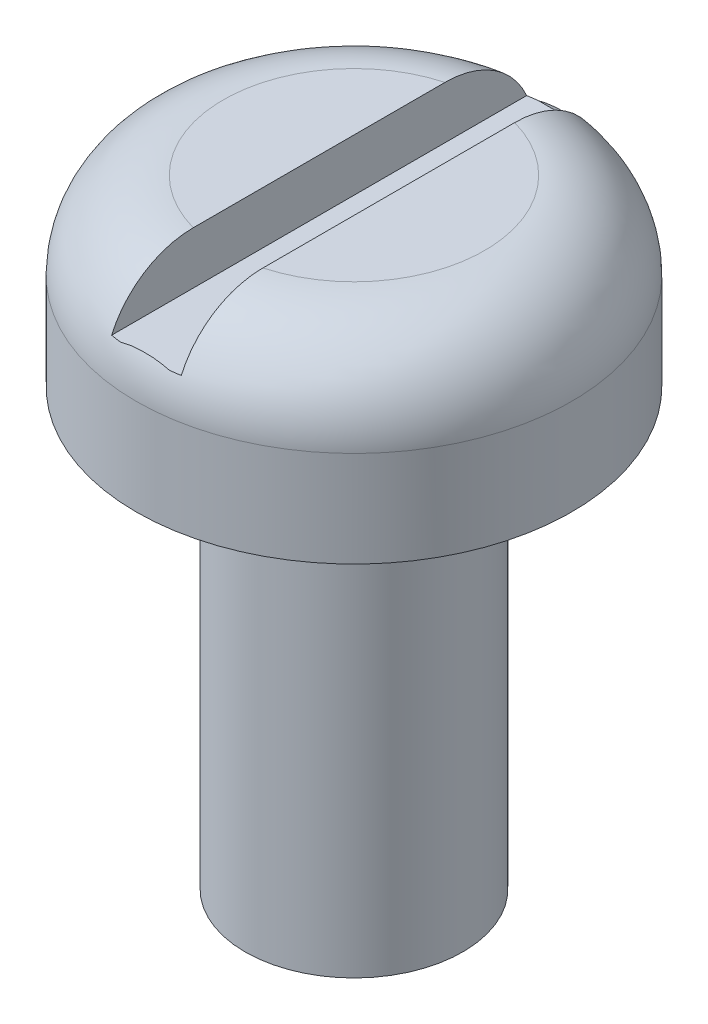
from build123d import *

# Parameters (mm, degrees)
HEAD_EDGE_FILLET_R1_R            = 1
SCREWDRIVER_SLOT_SKETCH_W        = 0.8
SCREWDRIVER_SLOT_SKETCH_H        = 4.8
SCREWDRIVER_SLOT_0_8_X_0_6_DEPTH = 0.6


with BuildPart() as part:
    # Bolt Profile Sketch → Bolt Body Ø2.5 Shank Ø5 Head (revolve)
    with BuildSketch(Plane.XY, mode=Mode.PRIVATE) as bolt_body_2_5_shank_5_head_sk:
        Polygon((0, -5), (1.25, -5), (1.25, 0), (2.5, 0), (2.5, 2.1), (0, 2.1), align=None)
    revolve(bolt_body_2_5_shank_5_head_sk.sketch.rotate(Axis((0, 4.110962567, 0), (0, -1, 0)), 90), axis=Axis((0, 4.110962567, 0), (0, -1, 0)))

    # Head Edge Fillet R1
    head_edge_fillet_r1_edges = [part.edges().sort_by_distance(p)[0] for p in [
        (0, 2.1, -2.5),
    ]]
    fillet(head_edge_fillet_r1_edges, radius=HEAD_EDGE_FILLET_R1_R)

    # Screwdriver Slot Sketch → Screwdriver Slot 0.8 x 0.6 (cut)
    with BuildSketch(Plane(origin=(0, 2.1, 0), x_dir=(1, 0, 0), z_dir=(0, 1, 0))):
        Rectangle(SCREWDRIVER_SLOT_SKETCH_W, SCREWDRIVER_SLOT_SKETCH_H)
    extrude(amount=-SCREWDRIVER_SLOT_0_8_X_0_6_DEPTH, mode=Mode.SUBTRACT)


solid = part.part
